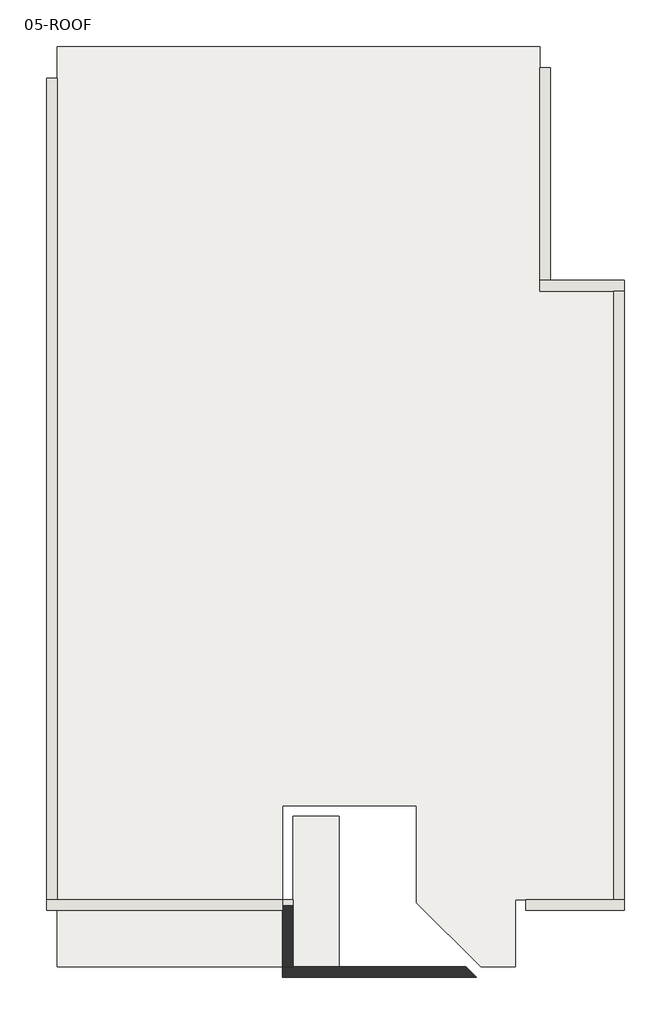
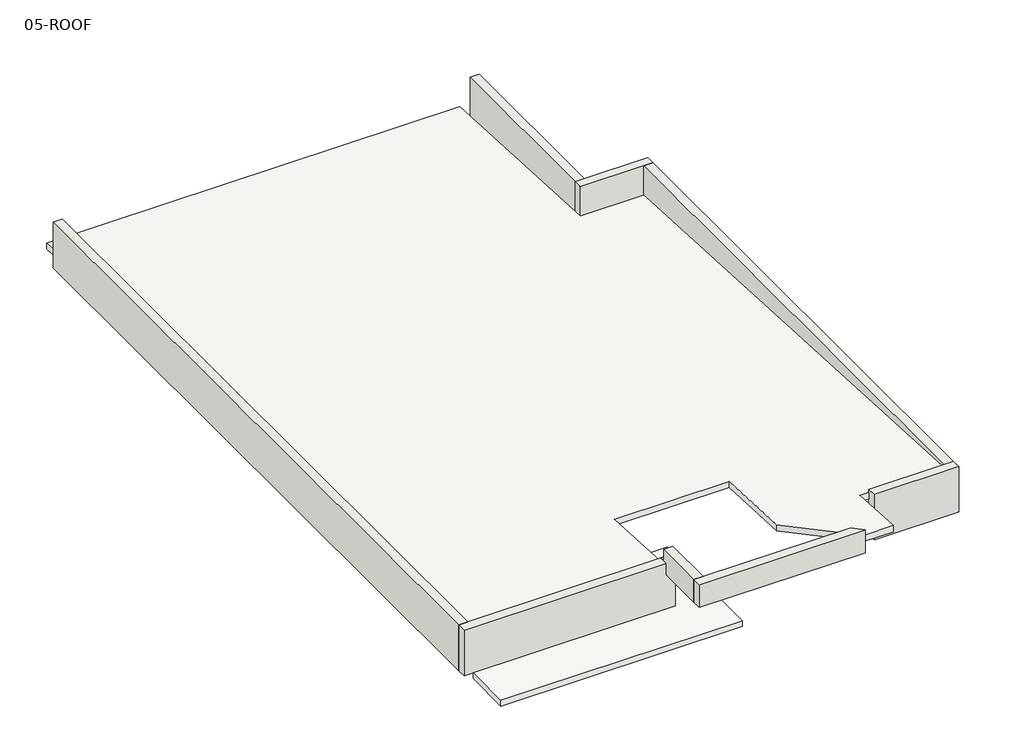
# One storey: 8 walls, 1 roof, 1 slab.
"""IFC4 building model written with IfcOpenShell, lengths in millimetres."""

from ifc_helpers import new_model, si_unit, frame, origin, place, context, project, spatial, polyline, outline, extrude, faceted_brep, element, save

model = new_model("IFC4")

# Units and contexts
model_context = context("Model", 3, world=origin())
ifc_project = project(units=[si_unit("LENGTHUNIT", "METRE", prefix="MILLI")], contexts=[model_context])

# Site, building, storey
site = spatial("IfcSite", under=ifc_project)
building = spatial("IfcBuilding", under=site)
storey = spatial("IfcBuildingStorey", under=building, Name="05-ROOF", Elevation=4350.0)

# Roof
placement = place(None, origin())
element("IfcRoof", 1, ObjectType="01-roof", at=placement, inside=storey, context=model_context, shape_type="Brep", body=[
    faceted_brep([(-8660.4564803, -12397.5265, 5301.201194), (-8660.4564803, 5752.4735, 4350.0), (1614.5435197, 5752.4735, 4350.0), (1614.5435197, 552.4735, 4622.5204523), (3189.5435197, 552.4735, 4622.5204523), (3189.5435197, -12397.5265, 5301.201194), (1089.5435197, -12397.5265, 5301.201194), (1089.5435197, -13822.5265, 5375.8822795), (357.7415713, -13822.5265, 5375.8822795), (-1010.4564803, -12454.3284484, 5304.178058), (-1010.4564803, -10397.5265, 5196.3856354), (-3860.4564803, -10397.5265, 5196.3856354), (-3860.4564803, -12397.5265, 5301.201194), (-8660.4564803, 5752.4735, 4510.2195754), (-8660.4564803, -12397.5265, 5461.4207693), (-3860.4564803, -12397.5265, 5461.4207693), (-3860.4564803, -10397.5265, 5356.6052108), (-1010.4564803, -10397.5265, 5356.6052108), (-1010.4564803, -12454.3284484, 5464.3976333), (357.7415713, -13822.5265, 5536.1018548), (1089.5435197, -13822.5265, 5536.1018548), (1089.5435197, -12397.5265, 5461.4207693), (3189.5435197, -12397.5265, 5461.4207693), (3189.5435197, 552.4735, 4782.7400276), (1614.5435197, 552.4735, 4782.7400276), (1614.5435197, 5752.4735, 4510.2195754)], [[[0, 1, 2, 3, 4, 5, 6, 7, 8, 9, 10, 11, 12]], [[13, 14, 15, 16, 17, 18, 19, 20, 21, 22, 23, 24, 25]], [[1, 13, 25, 2]], [[14, 13, 1, 0]], [[25, 24, 3, 2]], [[24, 23, 4, 3]], [[23, 22, 5, 4]], [[22, 21, 6, 5]], [[21, 20, 7, 6]], [[20, 19, 8, 7]], [[19, 18, 9, 8]], [[18, 17, 10, 9]], [[17, 16, 11, 10]], [[16, 15, 12, 11]], [[15, 14, 0, 12]]]),
])

# Slab
element("IfcSlab", 2, ObjectType="02-roof slab", at=placement, inside=storey, context=model_context, shape_type="SweptSolid", body=[
    extrude(outline(polyline([(-8660.4564803, -12622.5265), (-3635.4564803, -12622.5265), (-3635.4564803, -10622.5265), (-2660.4564803, -10622.5265), (-2660.4564803, -13822.5265), (-8660.4564803, -13822.5265), (-8660.4564803, -12622.5265)])), frame((0.0, 0.0, 4200.0), z_axis=(0.0, 0.0, 1.0), x_axis=(1.0, 0.0, 0.0)), (0.0, 0.0, 1.0), 150.0),
])

# Walls
element("IfcWall", 3, ObjectType="01-225 wall", at=placement, inside=storey, context=model_context, shape_type="Brep", body=[
    faceted_brep([(39.5435197, -13822.5265, 5250.0), (-3635.4564803, -13822.5265, 5250.0), (-3860.4564803, -13822.5265, 5250.0), (-3860.4564803, -13822.5265, 5850.0), (-3635.4564803, -13822.5265, 5850.0), (39.5435197, -13822.5265, 5850.0), (264.5435197, -14047.5265, 5250.0), (264.5435197, -14047.5265, 5850.0), (-3860.4564803, -14047.5265, 5850.0), (-3860.4564803, -14047.5265, 5250.0)], [[[0, 1, 2, 3, 4, 5]], [[6, 7, 8, 9]], [[2, 1, 0, 6, 9]], [[5, 4, 3, 8, 7]], [[0, 5, 7, 6]], [[3, 2, 9, 8]]]),
])
element("IfcWall", 4, ObjectType="01-225 wall", at=placement, inside=storey, context=model_context, shape_type="Brep", body=[
    faceted_brep([(-3860.4564803, -12397.5265, 5250.0), (-3860.4564803, -12622.5265, 5250.0), (-3860.4564803, -13822.5265, 5250.0), (-3860.4564803, -13822.5265, 5850.0), (-3860.4564803, -12510.0265, 5850.0), (-3860.4564803, -12510.0265, 5550.0), (-3860.4564803, -12397.5265, 5550.0), (-3635.4564803, -12397.5265, 5250.0), (-3635.4564803, -12397.5265, 5550.0), (-3635.4564803, -12510.0265, 5550.0), (-3635.4564803, -12510.0265, 5850.0), (-3635.4564803, -13822.5265, 5850.0), (-3635.4564803, -13822.5265, 5250.0), (-3635.4564803, -12622.5265, 5250.0)], [[[0, 1, 2, 3, 4, 5, 6]], [[7, 8, 9, 10, 11, 12, 13]], [[2, 1, 0, 7, 13, 12]], [[4, 3, 11, 10]], [[3, 2, 12, 11]], [[5, 4, 10, 9]], [[5, 9, 8, 6]], [[0, 6, 8, 7]]]),
])
element("IfcWall", 5, ObjectType="01-225 wall", at=placement, inside=storey, context=model_context, shape_type="Brep", body=[
    faceted_brep([(-3635.4564803, -12397.5265, 4350.0), (-3860.4564803, -12397.5265, 4350.0), (-8660.4564803, -12397.5265, 4350.0), (-8885.4564803, -12397.5265, 4350.0), (-8885.4564803, -12397.5265, 5550.0), (-8660.4564803, -12397.5265, 5550.0), (-3860.4564803, -12397.5265, 5550.0), (-3860.4564803, -12397.5265, 5250.0), (-3635.4564803, -12397.5265, 5250.0), (-3635.4564803, -12622.5265, 4350.0), (-3635.4564803, -12622.5265, 5250.0), (-3860.4564803, -12622.5265, 5250.0), (-3860.4564803, -12622.5265, 5550.0), (-8885.4564803, -12622.5265, 5550.0), (-8885.4564803, -12622.5265, 4350.0), (-8660.4564803, -12622.5265, 4350.0), (-3860.4564803, -12622.5265, 4350.0), (-3860.4564803, -12510.0265, 5550.0)], [[[0, 1, 2, 3, 4, 5, 6, 7, 8]], [[9, 10, 11, 12, 13, 14, 15, 16]], [[3, 2, 1, 0, 9, 16, 15, 14]], [[6, 5, 4, 13, 12, 17]], [[4, 3, 14, 13]], [[7, 11, 10, 8]], [[0, 8, 10, 9]], [[7, 6, 17, 12, 11]]]),
])
element("IfcWall", 6, ObjectType="01-225 wall", at=placement, inside=storey, context=model_context, shape_type="SweptSolid", body=[
    extrude(outline(polyline([(-8660.4564803, 5077.4735), (-8660.4564803, -12397.5265), (-8885.4564803, -12397.5265), (-8885.4564803, 5077.4735), (-8660.4564803, 5077.4735)])), frame((0.0, 0.0, 4350.0), z_axis=(0.0, 0.0, 1.0), x_axis=(1.0, 0.0, 0.0)), (0.0, 0.0, 1.0), 1200.0),
])
element("IfcWall", 7, ObjectType="01-225 wall", at=placement, inside=storey, context=model_context, shape_type="Brep", body=[
    faceted_brep([(1314.5435197, -12622.5265, 4350.0), (3414.5435197, -12622.5265, 4350.0), (3414.5435197, -12622.5265, 5550.0), (1314.5435197, -12622.5265, 5550.0), (1314.5435197, -12397.5265, 4350.0), (1314.5435197, -12397.5265, 5550.0), (3189.5435197, -12397.5265, 5550.0), (3414.5435197, -12397.5265, 5550.0), (3414.5435197, -12397.5265, 4350.0), (3189.5435197, -12397.5265, 4350.0)], [[[0, 1, 2, 3]], [[4, 5, 6, 7, 8, 9]], [[1, 0, 4, 9, 8]], [[3, 2, 7, 6, 5]], [[0, 3, 5, 4]], [[2, 1, 8, 7]]]),
])
element("IfcWall", 8, ObjectType="01-225 wall", at=placement, inside=storey, context=model_context, shape_type="Brep", body=[
    faceted_brep([(3414.5435197, 777.4735, 4350.0), (1839.5435197, 777.4735, 4350.0), (1614.5435197, 777.4735, 4350.0), (1614.5435197, 777.4735, 5550.0), (1839.5435197, 777.4735, 5550.0), (3414.5435197, 777.4735, 5550.0), (3414.5435197, 552.4735, 4350.0), (3414.5435197, 552.4735, 5550.0), (3189.5435197, 552.4735, 5550.0), (1614.5435197, 552.4735, 5550.0), (1614.5435197, 552.4735, 4350.0), (3189.5435197, 552.4735, 4350.0)], [[[0, 1, 2, 3, 4, 5]], [[6, 7, 8, 9, 10, 11]], [[2, 1, 0, 6, 11, 10]], [[5, 4, 3, 9, 8, 7]], [[3, 2, 10, 9]], [[0, 5, 7, 6]]]),
])
element("IfcWall", 9, ObjectType="01-225 wall", at=placement, inside=storey, context=model_context, shape_type="SweptSolid", body=[
    extrude(outline(polyline([(1839.5435197, 5302.4735), (1839.5435197, 777.4735), (1614.5435197, 777.4735), (1614.5435197, 5302.4735), (1839.5435197, 5302.4735)])), frame((0.0, 0.0, 4350.0), z_axis=(0.0, 0.0, 1.0), x_axis=(1.0, 0.0, 0.0)), (0.0, 0.0, 1.0), 1200.0),
])
element("IfcWall", 10, ObjectType="01-225 wall", at=placement, inside=storey, context=model_context, shape_type="SweptSolid", body=[
    extrude(outline(polyline([(3189.5435197, -12397.5265), (3189.5435197, 552.4735), (3414.5435197, 552.4735), (3414.5435197, -12397.5265), (3189.5435197, -12397.5265)])), frame((0.0, 0.0, 4350.0), z_axis=(0.0, 0.0, 1.0), x_axis=(1.0, 0.0, 0.0)), (0.0, 0.0, 1.0), 1200.0),
])

save(model, "model.ifc")

# Revit data of these elements
# Type "01-roof"
#   Description = "Generic Roof (Material By Category), 225mm thick"
#   Assembly Code = "B1020"
#   Type Mark = "G01"
# Type "02-roof slab"
#   Description = "Generic Floor (Material By Category), 12\" thick"
#   Assembly Code = "B1010"
#   Type Mark = "G01"
#   Function = 0
#   Layers, outside or top first: 150 mm "concrete floor" (function 1)
# Type "01-225 wall"
#   Description = "Generic Wall (Material By Category), 200mm thick"
#   Assembly Code = "B2010"
#   Type Mark = "G06"
#   Layers, outside or top first: 225 mm "01-225 wall paint" (function 1)
# Element 1 (IfcRoof, "01-roof")
#   built-in parameter 1001705 = 18.1631 (stored number, unit not read)
#   built-in parameter 1001710 = 33615
#   Phase Created = New Construction
# Element 2 (IfcSlab, "02-roof slab")
#   built-in parameter 1001955 = 1.5708 (stored number, unit not read)
#   Height Offset From Level = 0 mm
#   Phase Created = New Construction
#   Materials on its faces: "concrete floor"
# Elements 3, 4 (IfcWall, "01-225 wall")
#   built-in parameter 1001111 = 900 mm
#   Top Offset = 300 mm
#   Base Offset = 900 mm
#   wall height = 600 mm
#   Phase Created = New Construction
#   Base Constraint = 05-ROOF
#   Top Constraint = 06-PARAPET
#   Materials on its faces: "01-225 wall paint"
# Elements 5, 6, 7, 8, 9, 10 (IfcWall, "01-225 wall")
#   Top Offset = 0 mm
#   Base Offset = 0 mm
#   wall height = 1200 mm
#   Phase Created = New Construction
#   Base Constraint = 05-ROOF
#   Top Constraint = 06-PARAPET
#   Materials on its faces: "01-225 wall paint"
# Materials
#   "concrete floor": class "Generic", colour RGB 194 196 182, transparency 0, Cost = 0
#   "01-225 wall paint": class "Generic", colour RGB 242 242 255, transparency 0, Cost = 0
